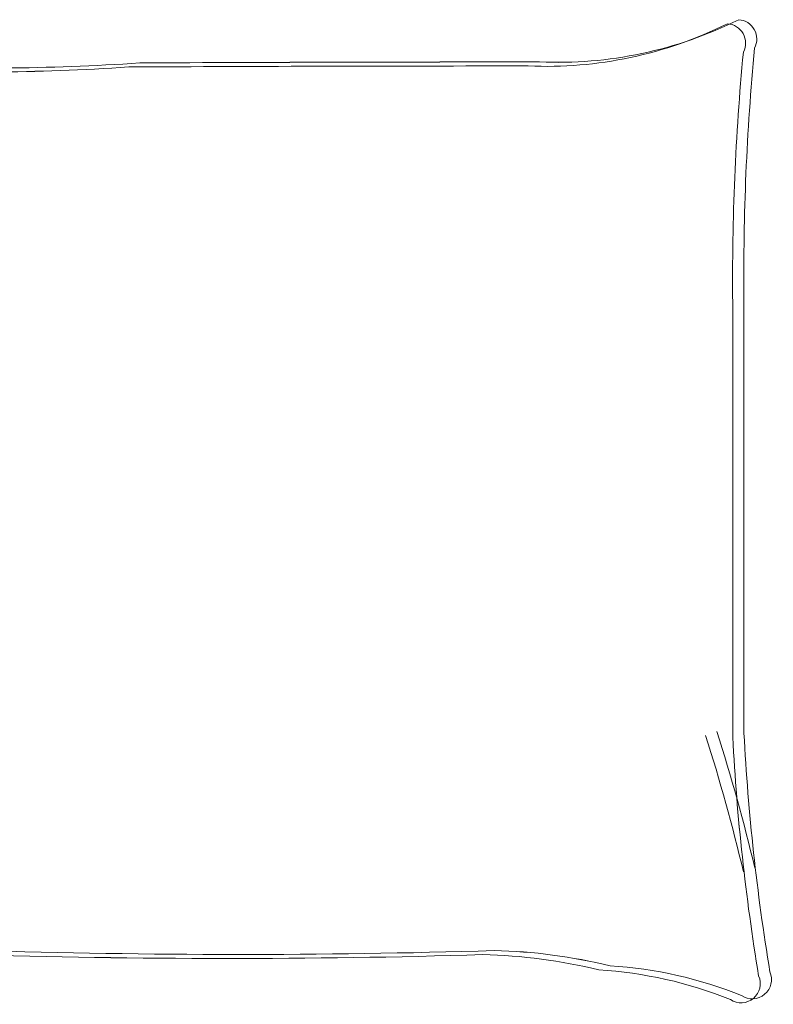
# Model space of a CAD drawing. Units: inches. Extents: x 1901 to 2863, y 888 to 2433.
# Tile 60 of 91: x 2073 to 2121, y 2130 to 2193. Entities that reach past the tile are written whole.
import ezdxf

# ---------------------------------------------------------------- set-up
doc = ezdxf.new("R2010")
doc.units = ezdxf.units.IN
doc.layers.add('A-FURN', color=8, linetype='Continuous', lineweight=18)

# ---------------------------------------------------------------- blocks, each defined once
blk = doc.blocks.new('BED-DOUBLE')
for p, q in [((31.896, 59.577), (28.246, 55.417)), ((31.896, 59.577), (28.246, 55.417)), ((33.854, 59.666), (31.896, 59.577, 4.346)), ((33.854, 59.666), (31.896, 59.577, 4.346)), ((32.591, 57.851), (31.896, 59.577)), ((32.591, 57.851), (31.896, 59.577)), ((31.178, 59.321), (27.529, 55.161)), ((31.178, 59.32), (27.529, 55.16)), ((33.137, 59.41), (31.178, 59.321, 4.346)), ((33.137, 59.41), (31.178, 59.32, 4.346)), ((31.873, 57.595), (31.178, 59.321)), ((31.873, 57.595), (31.178, 59.32)), ((0.026, 57.778), (0.026, 4.122)), ((0.744, 57.778), (30.62, 57.778)), ((0.744, 57.778), (30.62, 57.778)), ((32.243, 54.374), (32.591, 57.851)), ((32.243, 54.373), (32.591, 57.851)), ((19.351, 57.142), (15.827, 56.271)), ((19.351, 57.141), (15.827, 56.271)), ((18.898, 51.38), (19.351, 57.142)), ((18.898, 51.379), (19.351, 57.141)), ((31.525, 54.117), (31.873, 57.595)), ((31.525, 54.117), (31.873, 57.595)), ((3.615, 56.483), (3.506, 50.417)), ((3.615, 56.483), (3.506, 50.418)), ((3.615, 56.483), (7.22, 56.058)), ((3.615, 56.483), (7.22, 56.058)), ((6.502, 55.801), (9.388, 56.47)), ((6.502, 55.802), (9.388, 56.47)), ((7.22, 56.058), (10.106, 56.726)), ((7.22, 56.058), (10.106, 56.726)), ((9.388, 56.47), (10.563, 55.893)), ((9.388, 56.47), (10.563, 55.893)), ((14.025, 56.483), (10.015, 55.582)), ((14.025, 56.483), (10.015, 55.582)), ((10.106, 56.726), (11.28, 56.149)), ((10.106, 56.726), (11.28, 56.149)), ((15.827, 56.271), (14.025, 56.483)), ((15.827, 56.271), (14.025, 56.483)), ((18.633, 56.885), (15.109, 56.014)), ((18.633, 56.885), (15.109, 56.014)), ((18.18, 51.123), (18.633, 56.885)), ((18.18, 51.123), (18.633, 56.885)), ((2.897, 56.227), (2.788, 50.161)), ((2.897, 56.227), (2.788, 50.161)), ((2.897, 56.227), (6.502, 55.801)), ((2.897, 56.227), (6.502, 55.802)), ((13.307, 56.227), (9.297, 55.326)), ((13.307, 56.227), (9.297, 55.326)), ((15.109, 56.014), (13.307, 56.227)), ((15.109, 56.014), (13.307, 56.227)), ((9.297, 55.326), (6.289, 53.999)), ((9.297, 55.326), (6.289, 54)), ((10.015, 55.582), (7.007, 54.256)), ((10.015, 55.582), (7.007, 54.256)), ((27.529, 55.161), (25.096, 51.857)), ((27.529, 55.16), (25.096, 51.856)), ((28.246, 55.417), (25.814, 52.113)), ((28.246, 55.417), (25.814, 52.113)), ((31.873, 49.77), (31.525, 54.117)), ((31.873, 49.77), (31.525, 54.117)), ((32.591, 50.027), (32.243, 54.374)), ((32.591, 50.026), (32.243, 54.373)), ((25.814, 52.113), (23.554, 45.853)), ((25.814, 52.113), (23.554, 45.853)), ((3.506, 50.418), (3.598, 51.544)), ((3.506, 50.417), (3.598, 51.543)), ((3.598, 51.544), (4.19, 47.279)), ((3.598, 51.543), (4.19, 47.279)), ((25.096, 51.857), (22.837, 45.597)), ((25.096, 51.856), (22.837, 45.597)), ((2.788, 50.161), (2.881, 51.287)), ((2.788, 50.161), (2.881, 51.287)), ((2.881, 51.287), (3.472, 47.023)), ((2.881, 51.287), (3.472, 47.023)), ((18.806, 48.922), (18.18, 51.123)), ((18.806, 48.922), (18.18, 51.123)), ((19.523, 49.179), (18.898, 51.38)), ((19.523, 49.179), (18.898, 51.379)), ((32.394, 45.945), (31.873, 49.77)), ((32.394, 45.944), (31.873, 49.77)), ((33.112, 46.201), (32.591, 50.027)), ((33.112, 46.201), (32.591, 50.026)), ((18.322, 41.052), (18.806, 48.922)), ((18.322, 41.052), (18.806, 48.922)), ((19.039, 41.308), (19.523, 49.179)), ((19.039, 41.308), (19.523, 49.179)), ((3.472, 47.023), (4.991, 40.938)), ((3.472, 47.023), (4.991, 40.938)), ((4.19, 47.279), (5.709, 41.195)), ((4.19, 47.279), (5.709, 41.195)), ((23.554, 45.853), (20.261, 36.492)), ((23.554, 45.853), (20.261, 36.491)), ((33.437, 43.684), (32.394, 45.945)), ((33.437, 43.684), (32.394, 45.944)), ((34.155, 43.941), (33.112, 46.201)), ((34.155, 43.94), (33.112, 46.201)), ((22.837, 45.597), (19.543, 36.235)), ((22.837, 45.597), (19.543, 36.235)), ((88.998, 16.876), (88.998, 44.511)), ((88.998, 16.876), (88.998, 44.511)), ((89.716, 17.132), (89.716, 44.768)), ((89.716, 17.132), (89.716, 44.767)), ((4.151, 43.976), (3.482, 41.657)), ((4.151, 43.975), (3.482, 41.657)), ((4.869, 44.232), (4.2, 41.913)), ((4.869, 44.232), (4.2, 41.914)), ((34.85, 41.158), (34.155, 43.941)), ((34.85, 41.158), (34.155, 43.94)), ((34.132, 40.902), (33.437, 43.684)), ((34.132, 40.902), (33.437, 43.684)), ((3.482, 41.657), (2.875, 38.367)), ((3.482, 41.657), (2.875, 38.367)), ((4.2, 41.914), (3.593, 38.623)), ((4.2, 41.913), (3.593, 38.623)), ((17.573, 36.525), (18.322, 41.052)), ((17.573, 36.525), (18.322, 41.052)), ((18.291, 36.782), (19.039, 41.308)), ((18.291, 36.781), (19.039, 41.308)), ((27.551, 38.898), (32.591, 40.811)), ((27.551, 38.898), (32.591, 40.81)), ((31.873, 40.554), (34.132, 40.902)), ((31.873, 40.554), (34.132, 40.902)), ((32.591, 40.811), (34.85, 41.158)), ((32.591, 40.81), (34.85, 41.158)), ((26.834, 38.642), (31.873, 40.554)), ((26.834, 38.641), (31.873, 40.554)), ((20.261, 34.194), (27.551, 38.898)), ((20.261, 34.193), (27.551, 38.898)), ((2.875, 38.367), (2.897, 38.006)), ((2.875, 38.367), (2.897, 38.007)), ((3.593, 38.623), (3.615, 38.263)), ((3.593, 38.623), (3.615, 38.263)), ((3.615, 38.263), (4.088, 33.291)), ((3.615, 38.263), (4.088, 33.291)), ((19.543, 33.937), (26.834, 38.642)), ((19.543, 33.937), (26.834, 38.641)), ((2.897, 38.007), (3.371, 33.035)), ((2.897, 38.006), (3.371, 33.035)), ((18.82, 34.489), (17.378, 37.936)), ((18.82, 34.488), (17.378, 37.936)), ((19.538, 34.745), (18.096, 38.192)), ((19.538, 34.745), (18.096, 38.192)), ((18.993, 31.735), (18.82, 34.489)), ((18.993, 31.734), (18.82, 34.488)), ((19.71, 31.991), (19.538, 34.745)), ((19.71, 31.991), (19.538, 34.745)), ((4.088, 33.291), (3.542, 31.631)), ((4.088, 33.291), (3.542, 31.631)), ((3.371, 33.035), (2.824, 31.374)), ((3.371, 33.035), (2.824, 31.375)), ((16.706, 31.803), (19.71, 31.991)), ((16.706, 31.803), (19.71, 31.991)), ((2.824, 31.375), (8.859, 31.101)), ((2.824, 31.374), (8.859, 31.101)), ((3.542, 31.631), (9.577, 31.358)), ((3.542, 31.631), (9.577, 31.358)), ((9.577, 31.358), (13.182, 30.933)), ((9.577, 31.358), (13.182, 30.932)), ((13.922, 30.767), (15.988, 31.547)), ((13.922, 30.767), (15.988, 31.547)), ((14.64, 31.024), (16.706, 31.803)), ((14.64, 31.024), (16.706, 31.803)), ((15.988, 31.547), (18.993, 31.735)), ((15.988, 31.547), (18.993, 31.734)), ((8.859, 31.101), (12.464, 30.676)), ((8.859, 31.101), (12.464, 30.676)), ((12.464, 30.676), (13.922, 30.767)), ((12.464, 30.676), (13.922, 30.767)), ((13.182, 30.932), (14.64, 31.024)), ((13.182, 30.933), (14.64, 31.024)), ((8.132, 29.785), (11.704, 30.434)), ((8.132, 29.784), (11.704, 30.434)), ((8.85, 30.041), (12.422, 30.69)), ((8.85, 30.041), (12.422, 30.69)), ((11.704, 30.434), (13.165, 30.434)), ((11.704, 30.434), (13.165, 30.434)), ((12.422, 30.69), (13.883, 30.69)), ((12.422, 30.69), (13.883, 30.69)), ((13.165, 30.434), (15.275, 29.785)), ((13.165, 30.434), (15.275, 29.784)), ((13.883, 30.69), (15.993, 30.041)), ((13.883, 30.69), (15.993, 30.041)), ((2.126, 29.136), (8.132, 29.785)), ((2.126, 29.135), (8.132, 29.784)), ((2.844, 29.392), (8.85, 30.041)), ((2.844, 29.392), (8.85, 30.041)), ((15.275, 29.785), (18.286, 29.785)), ((15.275, 29.784), (18.286, 29.784)), ((15.993, 30.041), (19.003, 30.041)), ((15.993, 30.041), (19.003, 30.041)), ((18.286, 29.785), (18.286, 27.026)), ((18.286, 29.784), (18.286, 27.025)), ((19.003, 30.041), (19.003, 27.282)), ((19.003, 30.041), (19.003, 27.282)), ((2.775, 27.513), (2.126, 29.136)), ((2.775, 27.512), (2.126, 29.135)), ((3.493, 27.769), (2.844, 29.392)), ((3.493, 27.769), (2.844, 29.392)), ((3.331, 22.777), (3.493, 27.769)), ((3.331, 22.778), (3.493, 27.769)), ((18.898, 21.983), (19.351, 27.745)), ((18.898, 21.983), (19.351, 27.745)), ((2.613, 22.521), (2.775, 27.513)), ((2.613, 22.521), (2.775, 27.512)), ((18.286, 27.026), (17.061, 23.495)), ((18.286, 27.025), (17.061, 23.495)), ((19.003, 27.282), (17.779, 23.752)), ((19.003, 27.282), (17.779, 23.751)), ((18.18, 21.727), (18.633, 27.489)), ((18.18, 21.727), (18.633, 27.488)), ((3.331, 22.417), (3.331, 22.778)), ((3.331, 22.416), (3.331, 22.777)), ((2.613, 22.16), (2.613, 22.521)), ((2.613, 22.16), (2.613, 22.521)), ((3.425, 18.914), (2.613, 22.16)), ((3.425, 18.914), (2.613, 22.16)), ((4.142, 19.171), (3.331, 22.417)), ((4.142, 19.17), (3.331, 22.416)), ((19.523, 19.782), (18.898, 21.983)), ((19.523, 19.782), (18.898, 21.983)), ((18.806, 19.526), (18.18, 21.727)), ((18.806, 19.526), (18.18, 21.727)), ((3.749, 13.558), (4.886, 19.726)), ((3.749, 13.558), (4.886, 19.725)), ((4.467, 13.815), (5.603, 19.982)), ((4.467, 13.814), (5.603, 19.982)), ((18.322, 11.656), (18.806, 19.526)), ((18.322, 11.655), (18.806, 19.526)), ((19.039, 11.912), (19.523, 19.782)), ((19.039, 11.912), (19.523, 19.782)), ((4.236, 16.642), (3.425, 18.914)), ((4.236, 16.642), (3.425, 18.914)), ((4.954, 16.898), (4.142, 19.171)), ((4.954, 16.898), (4.142, 19.17)), ((4.142, 9.522), (4.467, 13.815)), ((4.142, 9.522), (4.467, 13.814)), ((3.425, 9.265), (3.749, 13.558)), ((3.425, 9.265), (3.749, 13.558)), ((18.291, 7.385), (19.039, 11.912)), ((18.291, 7.385), (19.039, 11.912)), ((19.039, 11.912), (19.402, 10.639)), ((19.039, 11.912), (19.402, 10.64)), ((17.573, 7.129), (18.322, 11.656)), ((17.573, 7.128), (18.322, 11.655)), ((18.322, 11.656), (18.684, 10.383)), ((18.322, 11.655), (18.684, 10.383)), ((18.684, 10.383), (19.496, 4.661)), ((18.684, 10.383), (19.496, 4.661)), ((19.402, 10.64), (20.214, 4.917)), ((19.402, 10.639), (20.214, 4.917)), ((4.122, 9.403), (4.142, 9.522)), ((4.122, 9.404), (4.142, 9.522)), ((4.492, 4.597), (4.122, 9.404)), ((4.492, 4.597), (4.122, 9.403)), ((3.404, 9.147), (3.425, 9.265)), ((3.404, 9.147), (3.425, 9.265)), ((3.774, 4.341), (3.404, 9.147)), ((3.774, 4.341), (3.404, 9.147)), ((10.798, 5.891), (7.714, 7.027)), ((10.798, 5.891), (7.714, 7.027)), ((10.08, 5.635), (6.996, 6.771)), ((10.08, 5.634), (6.996, 6.771)), ((14.857, 5.242), (10.798, 5.891)), ((14.857, 5.242), (10.798, 5.891)), ((4.467, 4.592), (8.039, 5.242)), ((4.467, 4.593), (8.038, 5.242)), ((8.038, 5.242), (10.961, 4.755)), ((8.039, 5.242), (10.961, 4.755)), ((14.139, 4.986), (10.08, 5.635)), ((14.139, 4.985), (10.08, 5.634)), ((10.243, 4.498), (11.379, 5.148)), ((10.243, 4.499), (11.379, 5.148)), ((10.961, 4.755), (12.097, 5.404)), ((10.961, 4.755), (12.097, 5.404)), ((15.925, 5.31), (14.139, 4.985)), ((15.924, 5.31), (14.139, 4.986)), ((16.642, 5.567), (14.857, 5.242)), ((16.642, 5.566), (14.857, 5.242)), ((19.496, 4.661), (15.924, 5.31)), ((19.496, 4.661), (15.925, 5.31)), ((20.214, 4.917), (16.642, 5.567)), ((20.214, 4.917), (16.642, 5.566)), ((3.749, 4.336), (7.321, 4.986)), ((3.749, 4.336), (7.321, 4.985)), ((7.321, 4.986), (10.243, 4.499)), ((7.321, 4.985), (10.243, 4.498))]:
    blk.add_line(p, q)
for centre, radius, start, end in [((77.121, 85.469), 25.896, 267.47137, 296.46809), ((77.121, 85.469), 25.896, 267.47137, 296.46809), ((77.839, 85.726), 25.896, 267.47137, 296.46809), ((77.839, 85.725), 25.896, 267.47137, 296.46809), ((88.578, 61.052), 1.238, 332.65876, 86.02002), ((88.578, 61.052), 1.238, 332.65876, 86.02002), ((89.295, 61.309), 1.238, 332.65876, 86.02002), ((89.295, 61.308), 1.238, 332.65876, 86.02002), ((238.36, 46.167), 149.37, 174.4998, 180.63509), ((238.36, 46.167), 149.37, 174.4998, 180.63509), ((239.077, 46.423), 149.37, 174.4998, 180.63509), ((239.077, 46.423), 149.37, 174.4998, 180.63509), ((-6.729, 57.848), 40.624, 349.87628, 2.56571), ((-6.729, 57.847), 40.624, 349.87628, 2.56571), ((41.517, 204.859), 145.395, 266.97912, 273.83645), ((41.517, 204.859), 145.395, 266.97912, 273.83645), ((76.173, -5062.226), 5121.824, 90.002168, 90.286888), ((76.173, -5062.226), 5121.824, 90.002168, 90.286888), ((76.89, -5061.969), 5121.824, 90.002168, 90.286888), ((76.89, -5061.97), 5121.824, 90.002168, 90.286888), ((-7.447, 57.591), 40.624, 349.87628, 2.56571), ((-7.447, 57.591), 40.624, 349.87628, 2.56571), ((40.799, 204.603), 145.395, 266.97912, 273.83645), ((40.799, 204.602), 145.395, 266.97912, 273.83645), ((39.397, 49.077), 6.988, 168.6608, 203.73842), ((39.397, 49.076), 6.988, 168.6608, 203.73842), ((40.115, 49.333), 6.988, 168.6608, 203.73842), ((40.115, 49.333), 6.988, 168.6608, 203.73842), ((2.408, 35.198), 33.294, 10.66171, 19.88058), ((2.408, 35.198), 33.294, 10.66171, 19.88058), ((1.69, 34.942), 33.294, 10.66171, 19.88058), ((1.69, 34.941), 33.294, 10.66171, 19.88058), ((176.248, 20.155), 144.857, 171.78449, 186.90062), ((176.248, 20.155), 144.857, 171.78449, 186.90062), ((34.202, 41.097), 0.207, 250.24637, 1.13765), ((34.202, 41.097), 0.207, 250.24637, 1.13765), ((34.92, 41.353), 0.207, 250.24637, 1.13765), ((34.92, 41.353), 0.207, 250.24637, 1.13765), ((175.53, 19.899), 144.857, 171.78449, 186.90062), ((175.53, 19.899), 144.857, 171.78449, 186.90062), ((204.426, 23.944), 185.219, 176.08655, 186.78213), ((204.426, 23.944), 185.219, 176.08655, 186.78213), ((205.143, 24.201), 185.219, 176.08655, 186.78213), ((205.143, 24.2), 185.219, 176.08655, 186.78213), ((226.234, 24.277), 136.704, 182.99578, 189.40907), ((226.234, 24.277), 136.704, 182.99578, 189.40907), ((225.516, 24.021), 136.704, 182.99578, 189.40907), ((225.516, 24.02), 136.704, 182.99578, 189.40907), ((35.744, -187.624), 190.991, 88.4762, 91.00819), ((35.744, -187.625), 190.991, 88.4762, 91.00819), ((57.571, 544.554), 541.514, 268.22771, 271.71854), ((57.571, 544.554), 541.514, 268.22771, 271.71854), ((73.178, -29.981), 33.271, 76.06484, 88.91125), ((73.178, -29.982), 33.271, 76.06484, 88.91125), ((23.307, 95.835), 93.531, 268.72178, 275.60397), ((23.307, 95.835), 93.531, 268.72178, 275.60397), ((35.026, -187.881), 190.991, 88.4762, 91.00819), ((35.026, -187.881), 190.991, 88.4762, 91.00819), ((56.853, 544.298), 541.514, 268.22771, 271.71854), ((56.853, 544.297), 541.514, 268.22771, 271.71854), ((72.461, -30.238), 33.271, 76.06484, 88.91125), ((72.461, -30.238), 33.271, 76.06484, 88.91125), ((22.589, 95.579), 93.531, 268.72178, 275.60397), ((22.589, 95.579), 93.531, 268.72178, 275.60397), ((78.928, -24.355), 26.454, 67.97508, 86.652), ((78.928, -24.355), 26.454, 67.97508, 86.652), ((79.646, -24.098), 26.454, 67.97508, 86.652), ((79.646, -24.098), 26.454, 67.97508, 86.652), ((90.247, 1.441), 1.223, 236.17358, 23.47814), ((90.247, 1.441), 1.223, 236.17358, 23.47814), ((89.529, 1.185), 1.223, 236.17358, 23.47814), ((89.529, 1.184), 1.223, 236.17358, 23.47814)]:
    blk.add_arc(centre, radius, start, end)

msp = doc.modelspace()

# ---------------------------------------------------------------- linework, layer by layer
at = {"layer": 'A-FURN'}
for centre in [(2002.804, 2110.628), (2002.804, 2110.628), (2003.521, 2110.884), (2003.521, 2110.884)]:
    msp.add_arc(centre, 119.527, 13.38322, 17.70533, dxfattribs=at)

# ---------------------------------------------------------------- block references
msp.add_blockref('BED-DOUBLE', (2029.4, 2130), dxfattribs=at)

doc.saveas('drawing.dxf')
